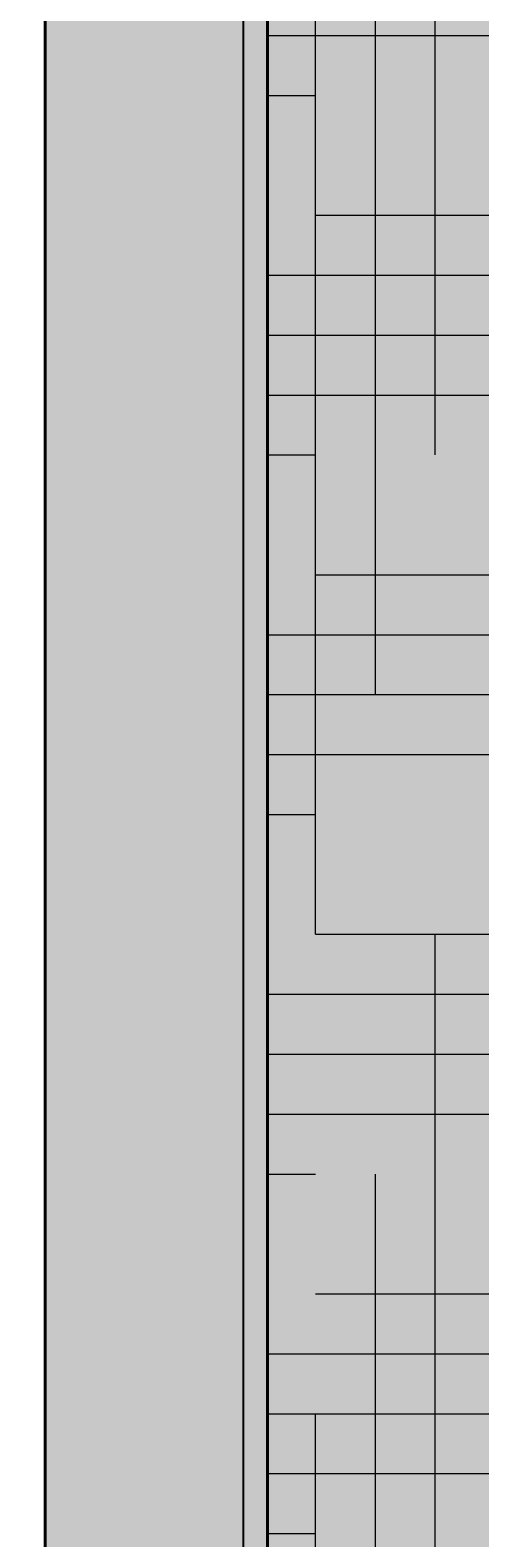
# Model space of a CAD drawing. Units: feet. Extents: x 2695 to 2912, y 795 to 1139.
# Tile 6 of 83: x 2710 to 2722, y 835 to 875. Entities that reach past the tile are written whole.
import ezdxf

# ---------------------------------------------------------------- set-up
doc = ezdxf.new("R2010")
doc.units = ezdxf.units.FT
for name, color, linetype, lineweight in [('A-ANNO-DIMS', 2, 'Continuous', 18), ('A-ELEV', 7, 'Continuous', 35), ('A-ELEV-PATT', 252, 'Continuous', 13)]:
    doc.layers.add(name, color=color, linetype=linetype, lineweight=lineweight)
doc.styles.get("Standard").update_dxf_attribs({"font": 'arial.ttf'})
doc.dimstyles.get("Standard").update_dxf_attribs({"dimtxt": 0.18, "dimasz": 0.18, "dimexe": 0.18, "dimexo": 0.0625, "dimgap": 0.09, "dimtad": 0, "dimtih": 1, "dimtoh": 1, "dimdec": 1, "dimzin": 0, "dimdsep": 46, "dimlunit": 3, "dimtxsty": 'Standard', "dimcen": 0.09, "dimadec": 0, "dimazin": 0, "dimtfac": 1, "dimtdec": 1, "dimtofl": 0, "dimtmove": 0, "dimatfit": 3, "dimfxl": 1, "dimtolj": 1, "dimtzin": 0, "dimarcsym": 0})

# ---------------------------------------------------------------- blocks, each defined once
blk = doc.blocks.new('*D2')
at = {"layer": 'A-ANNO-DIMS', "color": 0, "lineweight": -2, "transparency": 16777216}
for p, q in [((2724.189, 874.795), (2724.189, 794.976)), ((2716.536, 810.868), (2716.536, 794.976)), ((2716.716, 795.156), (2719.97, 795.156)), ((2724.009, 795.156), (2720.756, 795.156))]:
    blk.add_line(p, q, dxfattribs=at)
at = {"layer": 'A-ANNO-DIMS', "color": 0, "transparency": 16777216}
for points in [[(2716.716, 795.186), (2716.716, 795.126), (2716.536, 795.156)], [(2724.009, 795.186), (2724.009, 795.126), (2724.189, 795.156)]]:
    blk.add_solid(points, dxfattribs=at)
at = {"layer": 'Defpoints', "color": 0, "transparency": 16777216}
for p in [(2724.189, 874.857), (2716.536, 810.931), (2724.189, 795.156)]:
    blk.add_point(p, dxfattribs=at)
at = {"layer": 'A-ANNO-DIMS', "color": 0, "transparency": 16777216, "insert": (2720.363, 795.156), "char_height": 0.18, "attachment_point": 5}
blk.add_mtext('\\A1;7.653', dxfattribs=at)
blk = doc.blocks.new('*D12')
at = {"layer": 'A-ANNO-DIMS', "color": 0, "lineweight": -2, "transparency": 16777216}
for p, q in [((2710.574, 1122.931), (2694.681, 1122.931)), ((2694.861, 1122.751), (2694.861, 967.113)), ((2694.861, 811.111), (2694.861, 966.749)), ((2710.574, 810.931), (2694.681, 810.931))]:
    blk.add_line(p, q, dxfattribs=at)
at = {"layer": 'A-ANNO-DIMS', "color": 0, "transparency": 16777216}
for points in [[(2694.831, 1122.751), (2694.891, 1122.751), (2694.861, 1122.931)], [(2694.831, 811.111), (2694.891, 811.111), (2694.861, 810.931)]]:
    blk.add_solid(points, dxfattribs=at)
at = {"layer": 'Defpoints', "color": 0, "transparency": 16777216}
for p in [(2694.861, 1122.931), (2710.636, 1122.931), (2710.636, 810.931)]:
    blk.add_point(p, dxfattribs=at)
at = {"layer": 'A-ANNO-DIMS', "color": 0, "transparency": 16777216, "insert": (2694.861, 966.931), "char_height": 0.18, "attachment_point": 5}
blk.add_mtext('\\A1;312', dxfattribs=at)
blk = doc.blocks.new('*D23')
at = {"layer": 'A-ANNO-DIMS', "color": 0, "lineweight": -2, "transparency": 16777216}
for p, q in [((2715.885, 936.868), (2715.885, 794.976)), ((2730.708, 936.868), (2730.708, 794.976)), ((2716.065, 795.156), (2722.842, 795.156)), ((2730.528, 795.156), (2723.752, 795.156))]:
    blk.add_line(p, q, dxfattribs=at)
at = {"layer": 'A-ANNO-DIMS', "color": 0, "transparency": 16777216}
for points in [[(2716.065, 795.186), (2716.065, 795.126), (2715.885, 795.156)], [(2730.528, 795.186), (2730.528, 795.126), (2730.708, 795.156)]]:
    blk.add_solid(points, dxfattribs=at)
at = {"layer": 'Defpoints', "color": 0, "transparency": 16777216}
for p in [(2715.885, 936.931), (2730.708, 936.931), (2730.708, 795.156)]:
    blk.add_point(p, dxfattribs=at)
at = {"layer": 'A-ANNO-DIMS', "color": 0, "transparency": 16777216, "insert": (2723.297, 795.156), "char_height": 0.18, "attachment_point": 5}
blk.add_mtext('\\A1;14.823', dxfattribs=at)

msp = doc.modelspace()

# ---------------------------------------------------------------- hatches: boundary and pattern name
at = {"layer": 'A-ELEV-PATT'}
h = msp.add_hatch(color=256, dxfattribs=at)
h.set_gradient(color1=(255, 255, 255), tint=1)
h.paths.add_polyline_path([(2770.6361, 1122.9306), (2710.6361, 1122.9306), (2710.6361, 1118.4096), (2770.6361, 1118.4096)])
h.paths.add_polyline_path([(2890.6361, 1107.8588), (2770.6361, 1107.8588), (2770.6361, 1103.3378), (2890.6361, 1103.3378)])
h.paths.add_polyline_path([(2890.6361, 1062.9306), (2710.6361, 1062.9306), (2710.6361, 1056.9306), (2710.6361, 936.9306), (2710.6361, 924.3105), (2716.5358, 924.3105), (2890.6361, 924.3105), (2890.6361, 936.9306), (2715.8852, 936.9306), (2715.8852, 1050.3105), (2890.6361, 1050.3105)])
h.paths.add_polyline_path([(2716.5358, 924.3105), (2710.6361, 924.3105), (2710.6361, 810.9306), (2716.5358, 810.9306)])
h = msp.add_hatch(color=256, dxfattribs=at)
h.set_gradient(color1=(255, 255, 255))
h.paths.add_polyline_path([(2770.6361, 924.3105), (2716.5358, 924.3105), (2716.5358, 810.9306), (2770.6361, 810.9306)])
h.paths.add_polyline_path([(2758.1515, 902.577), (2758.1515, 874.8571), (2724.1893, 874.8571), (2724.1893, 902.577)], flags=16)
h.paths.add_polyline_path([(2756.1515, 900.577), (2756.1515, 876.8571), (2726.1893, 876.8571), (2726.1893, 900.577)], flags=0)
h.paths.add_polyline_path([(2740.7302, 900.577), (2741.6105, 900.577), (2741.6105, 876.8571), (2740.7302, 876.8571)], flags=0)
h = msp.add_hatch(dxfattribs=at)
h.set_pattern_fill('HOUND', color=256, style=0)
h.paths.add_polyline_path([(2770.6361, 924.3105), (2716.5358, 924.3105), (2716.5358, 810.9306), (2770.6361, 810.9306)])
h.paths.add_polyline_path([(2724.1893, 874.8571), (2724.1893, 902.577), (2758.1515, 902.577), (2758.1515, 874.8571)], flags=16)
h.paths.add_polyline_path([(2756.1515, 876.8571), (2726.1893, 876.8571), (2726.1893, 900.577), (2756.1515, 900.577)], flags=0)
h.paths.add_polyline_path([(2741.6105, 876.8571), (2740.7302, 876.8571), (2740.7302, 900.577), (2741.6105, 900.577)], flags=0)

# ---------------------------------------------------------------- linework, layer by layer
at = {"layer": 'A-ELEV'}
for p, q in [((2710.6361, 930.9306), (2710.6361, 810.9306)), ((2716.5358, 924.3105), (2716.5358, 810.9306))]:
    msp.add_line(p, q, dxfattribs=at)
for points in [[(2710.6361, 924.3105), (2716.5358, 924.3105), (2716.5358, 810.9306), (2710.6361, 810.9306)], [(2716.5358, 924.3105), (2770.6361, 924.3105), (2770.6361, 810.9306), (2716.5358, 810.9306)]]:
    msp.add_lwpolyline(points, close=True, dxfattribs=at)

# ---------------------------------------------------------------- dimensions: what is measured, and where the dimension line sits
at = {"layer": 'A-ANNO-DIMS'}
dim = msp.add_linear_dim(base=(2694.8611, 1122.9306), p1=(2710.6361, 810.9306), p2=(2710.6361, 1122.9306), angle=90, dimstyle='Standard', override={"dimdec": 0, "dimlfac": 1, "dimrnd": 0, "dimzin": 0, "dimdsep": 46, "dimlunit": 2}, dxfattribs=at)
dim.commit()
dim.dimension.update_dxf_attribs({"geometry": '*D12', "text_midpoint": (2694.8611, 966.9306)})
for base, p1, p2, picture, middle in [((2730.7081, 795.1556), (2715.8852, 936.9306), (2730.7081, 936.9306), '*D23', (2723.2967, 795.1556)), ((2724.18927, 795.15559), (2716.53582, 810.93059), (2724.18927, 874.85709), '*D2', (2720.36254, 795.15559))]:
    dim = msp.add_linear_dim(base=base, p1=p1, p2=p2, dimstyle='Standard', override={"dimdec": 3, "dimlfac": 1, "dimrnd": 0, "dimzin": 0, "dimdsep": 46, "dimlunit": 2}, dxfattribs=at)
    dim.commit()
    dim.dimension.update_dxf_attribs({"geometry": picture, "text_midpoint": middle})

doc.saveas('drawing.dxf')
